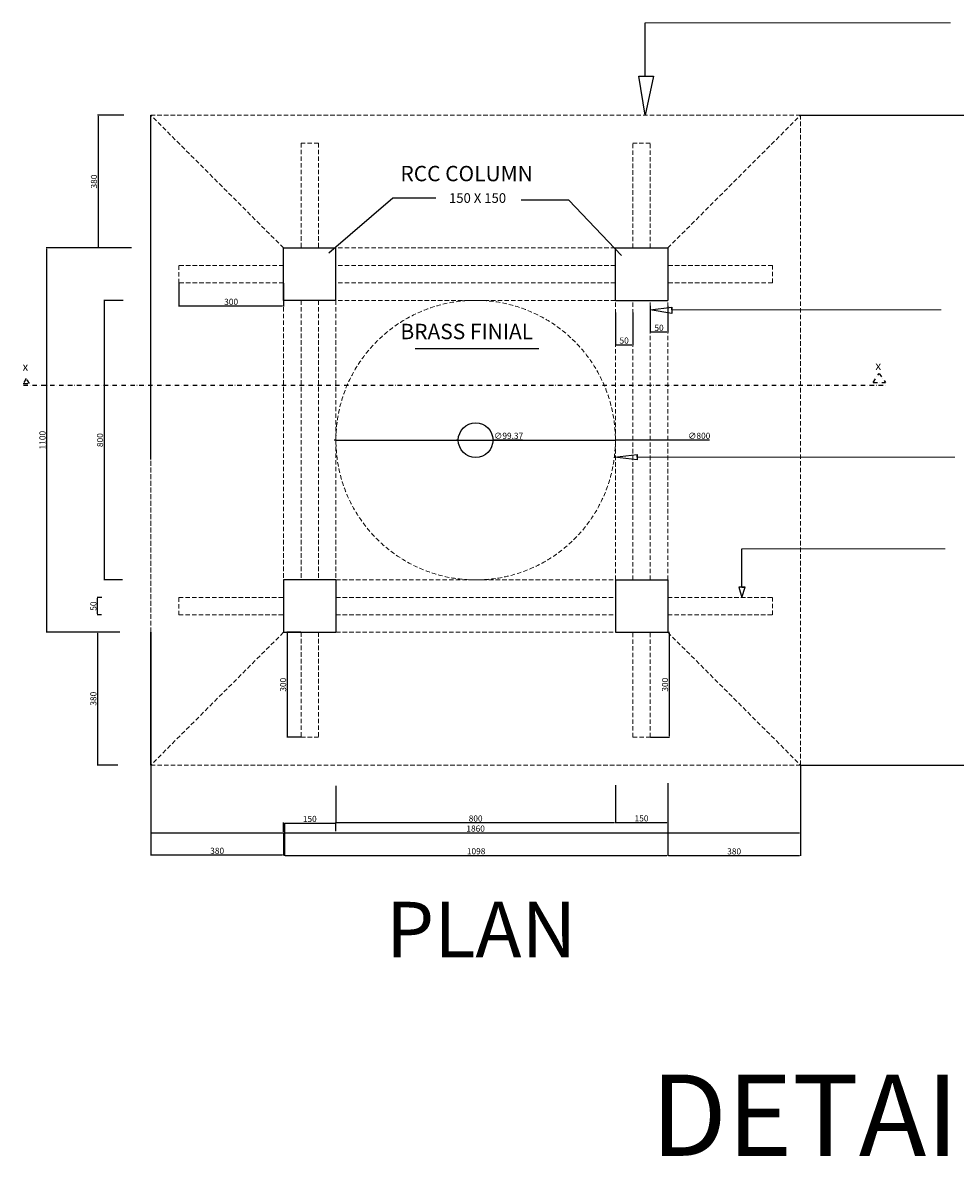
# Model space of a CAD drawing. Units: millimetres. Extents: x 498 to 8860, y -426 to 8717.
# Tile 1 of 9: x 498 to 3168, y -426 to 2821. Entities that reach past the tile are written whole.
import ezdxf

# ---------------------------------------------------------------- set-up
doc = ezdxf.new("R2010")
doc.units = ezdxf.units.MM
doc.linetypes.add('DASHDOT', pattern=[25.4, 12.7, -6.35, 0, -6.35])
doc.linetypes.add('DASHED', pattern=[19.05, 12.7, -6.35])
for name, color, linetype, lineweight in [('A-ANNO-DIMS', 2, 'Continuous', 18), ('A-ANNO-SYMB', 1, 'DASHDOT', 25), ('A-ANNO-TEXT', 3, 'Continuous', 18), ('A-DETL', 7, 'Continuous', 25), ('A-DETL-OVHD', 8, 'DASHED', 18)]:
    doc.layers.add(name, color=color, linetype=linetype, lineweight=lineweight)
doc.styles.get("Standard").update_dxf_attribs({"font": 'arial.ttf'})
doc.dimstyles.new('ISO-25', dxfattribs={"dimtxt": 17.5, "dimasz": 2.5, "dimexe": 1.25, "dimexo": 0.625, "dimtad": 1, "dimdec": 0, "dimtxsty": 'Standard', "dimcen": 2.5, "dimadec": 0, "dimazin": 0, "dimtfac": 1, "dimtdec": 0, "dimtmove": 0, "dimatfit": 3, "dimfxl": 1, "dimarcsym": 0})

# ---------------------------------------------------------------- blocks, each defined once
blk = doc.blocks.new('*D1')
at = {"layer": 'A-ANNO-DIMS', "color": 0, "lineweight": -2, "transparency": 16777216}
for p, q in [((944.7, 2075.6), (944.7, 2009.1)), ((1244.7, 2075.6), (1244.7, 2009.1)), ((947.2, 2010.4), (1242.2, 2010.4))]:
    blk.add_line(p, q, dxfattribs=at)
at = {"layer": 'A-ANNO-DIMS', "color": 0, "transparency": 16777216}
for points in [[(947.2, 2010.8), (947.2, 2009.9), (944.7, 2010.4)], [(1242.2, 2010.8), (1242.2, 2009.9), (1244.7, 2010.4)]]:
    blk.add_solid(points, dxfattribs=at)
at = {"layer": 'Defpoints', "color": 0, "transparency": 16777216}
for p in [(944.7, 2076.3), (1244.7, 2076.3), (1244.7, 2010.4)]:
    blk.add_point(p, dxfattribs=at)
at = {"layer": 'A-ANNO-DIMS', "color": 0, "transparency": 16777216, "insert": (1094.7, 2019.9), "char_height": 17.5, "attachment_point": 5}
blk.add_mtext('300', dxfattribs=at)
blk = doc.blocks.new('*D2')
at = {"layer": 'A-ANNO-DIMS', "color": 0, "lineweight": -2, "transparency": 16777216}
for p, q in [((724.4, 1176.3), (710.9, 1176.3)), ((712.2, 1128.8), (712.2, 1173.8)), ((723.9, 1126.3), (710.9, 1126.3))]:
    blk.add_line(p, q, dxfattribs=at)
at = {"layer": 'A-ANNO-DIMS', "color": 0, "transparency": 16777216}
for points in [[(711.8, 1173.8), (712.6, 1173.8), (712.2, 1176.3)], [(711.8, 1128.8), (712.6, 1128.8), (712.2, 1126.3)]]:
    blk.add_solid(points, dxfattribs=at)
at = {"layer": 'Defpoints', "color": 0, "transparency": 16777216}
for p in [(712.2, 1176.3), (725, 1176.3), (724.5, 1126.3)]:
    blk.add_point(p, dxfattribs=at)
at = {"layer": 'A-ANNO-DIMS', "color": 0, "transparency": 16777216, "insert": (702.6, 1151.3), "char_height": 17.5, "attachment_point": 5, "rotation": 90}
blk.add_mtext('50', dxfattribs=at)
blk = doc.blocks.new('*D3')
at = {"layer": 'A-ANNO-DIMS', "color": 0, "lineweight": -2, "transparency": 16777216}
for p, q in [((787.7, 2556.3), (712.6, 2556.3)), ((713.9, 2553.8), (713.9, 2178.8)), ((809.4, 2176.3), (712.6, 2176.3))]:
    blk.add_line(p, q, dxfattribs=at)
at = {"layer": 'A-ANNO-DIMS', "color": 0, "transparency": 16777216}
for points in [[(713.4, 2553.8), (714.3, 2553.8), (713.9, 2556.3)], [(713.4, 2178.8), (714.3, 2178.8), (713.9, 2176.3)]]:
    blk.add_solid(points, dxfattribs=at)
at = {"layer": 'Defpoints', "color": 0, "transparency": 16777216}
for p in [(788.4, 2556.3), (713.9, 2176.3), (810, 2176.3)]:
    blk.add_point(p, dxfattribs=at)
at = {"layer": 'A-ANNO-DIMS', "color": 0, "transparency": 16777216, "insert": (704.3, 2366.3), "char_height": 17.5, "attachment_point": 5, "rotation": 90}
blk.add_mtext('380', dxfattribs=at)
blk = doc.blocks.new('*D4')
at = {"layer": 'A-ANNO-DIMS', "color": 0, "lineweight": -2, "transparency": 16777216}
for p, q in [((775.7, 1076.3), (710.9, 1076.3)), ((712.2, 1073.8), (712.2, 698.8)), ((770.5, 696.3), (710.9, 696.3))]:
    blk.add_line(p, q, dxfattribs=at)
at = {"layer": 'A-ANNO-DIMS', "color": 0, "transparency": 16777216}
for points in [[(711.8, 1073.8), (712.6, 1073.8), (712.2, 1076.3)], [(711.8, 698.8), (712.6, 698.8), (712.2, 696.3)]]:
    blk.add_solid(points, dxfattribs=at)
at = {"layer": 'Defpoints', "color": 0, "transparency": 16777216}
for p in [(776.4, 1076.3), (712.2, 696.3), (771.2, 696.3)]:
    blk.add_point(p, dxfattribs=at)
at = {"layer": 'A-ANNO-DIMS', "color": 0, "transparency": 16777216, "insert": (702.6, 886.3), "char_height": 17.5, "attachment_point": 5, "rotation": 90}
blk.add_mtext('380', dxfattribs=at)
blk = doc.blocks.new('*D5')
at = {"layer": 'A-ANNO-DIMS', "color": 0, "lineweight": -2, "transparency": 16777216}
for p, q in [((739.8, 2176.3), (565.1, 2176.3)), ((566.3, 2173.8), (566.3, 1078.8)), ((775.7, 1076.3), (565.1, 1076.3))]:
    blk.add_line(p, q, dxfattribs=at)
at = {"layer": 'A-ANNO-DIMS', "color": 0, "transparency": 16777216}
for points in [[(565.9, 2173.8), (566.7, 2173.8), (566.3, 2176.3)], [(565.9, 1078.8), (566.7, 1078.8), (566.3, 1076.3)]]:
    blk.add_solid(points, dxfattribs=at)
at = {"layer": 'Defpoints', "color": 0, "transparency": 16777216}
for p in [(740.4, 2176.3), (566.3, 1076.3), (776.4, 1076.3)]:
    blk.add_point(p, dxfattribs=at)
at = {"layer": 'A-ANNO-DIMS', "color": 0, "transparency": 16777216, "insert": (556.8, 1626.3), "char_height": 17.5, "attachment_point": 5, "rotation": 90}
blk.add_mtext('1100', dxfattribs=at)
blk = doc.blocks.new('*D6')
at = {"layer": 'A-ANNO-DIMS', "color": 0, "lineweight": -2, "transparency": 16777216}
for p, q in [((1294.1, 1076.3), (1254, 1076.3)), ((1255.3, 1073.8), (1255.3, 778.8)), ((1294.1, 776.3), (1254, 776.3))]:
    blk.add_line(p, q, dxfattribs=at)
at = {"layer": 'A-ANNO-DIMS', "color": 0, "transparency": 16777216}
for points in [[(1254.9, 1073.8), (1255.7, 1073.8), (1255.3, 1076.3)], [(1254.9, 778.8), (1255.7, 778.8), (1255.3, 776.3)]]:
    blk.add_solid(points, dxfattribs=at)
at = {"layer": 'Defpoints', "color": 0, "transparency": 16777216}
for p in [(1294.7, 1076.3), (1255.3, 776.3), (1294.7, 776.3)]:
    blk.add_point(p, dxfattribs=at)
at = {"layer": 'A-ANNO-DIMS', "color": 0, "transparency": 16777216, "insert": (1245.7, 926.3), "char_height": 17.5, "attachment_point": 5, "rotation": 90}
blk.add_mtext('300', dxfattribs=at)
blk = doc.blocks.new('*D7')
at = {"layer": 'A-ANNO-DIMS', "color": 0, "lineweight": -2, "transparency": 16777216}
for p, q in [((2295.4, 1076.3), (2349.9, 1076.3)), ((2348.6, 1073.8), (2348.6, 778.8)), ((2295.4, 776.3), (2349.9, 776.3))]:
    blk.add_line(p, q, dxfattribs=at)
at = {"layer": 'A-ANNO-DIMS', "color": 0, "transparency": 16777216}
for points in [[(2348.2, 1073.8), (2349, 1073.8), (2348.6, 1076.3)], [(2348.2, 778.8), (2349, 778.8), (2348.6, 776.3)]]:
    blk.add_solid(points, dxfattribs=at)
at = {"layer": 'Defpoints', "color": 0, "transparency": 16777216}
for p in [(2294.7, 1076.3), (2294.7, 776.3), (2348.6, 776.3)]:
    blk.add_point(p, dxfattribs=at)
at = {"layer": 'A-ANNO-DIMS', "color": 0, "transparency": 16777216, "insert": (2339.1, 926.3), "char_height": 17.5, "attachment_point": 5, "rotation": 90}
blk.add_mtext('300', dxfattribs=at)
blk = doc.blocks.new('*D8')
at = {"layer": 'A-ANNO-DIMS', "color": 0, "lineweight": -2, "transparency": 16777216}
for p, q in [((2294.7, 2010.9), (2294.7, 1934.6)), ((2344.7, 2010.9), (2344.7, 1934.6)), ((2297.2, 1935.9), (2342.2, 1935.9))]:
    blk.add_line(p, q, dxfattribs=at)
at = {"layer": 'A-ANNO-DIMS', "color": 0, "transparency": 16777216}
for points in [[(2297.2, 1936.3), (2297.2, 1935.4), (2294.7, 1935.9)], [(2342.2, 1936.3), (2342.2, 1935.4), (2344.7, 1935.9)]]:
    blk.add_solid(points, dxfattribs=at)
at = {"layer": 'Defpoints', "color": 0, "transparency": 16777216}
for p in [(2294.7, 2011.5), (2344.7, 2011.5), (2344.7, 1935.9)]:
    blk.add_point(p, dxfattribs=at)
at = {"layer": 'A-ANNO-DIMS', "color": 0, "transparency": 16777216, "insert": (2319.7, 1945.4), "char_height": 17.5, "attachment_point": 5}
blk.add_mtext('50', dxfattribs=at)
blk = doc.blocks.new('*D9')
at = {"layer": 'A-ANNO-DIMS', "color": 0, "lineweight": -2, "transparency": 16777216}
for p, q in [((2194.7, 1991.4), (2194.7, 1898.2)), ((2244.7, 1991.4), (2244.7, 1898.2)), ((2197.2, 1899.5), (2242.2, 1899.5))]:
    blk.add_line(p, q, dxfattribs=at)
at = {"layer": 'A-ANNO-DIMS', "color": 0, "transparency": 16777216}
for points in [[(2197.2, 1899.9), (2197.2, 1899.1), (2194.7, 1899.5)], [(2242.2, 1899.9), (2242.2, 1899.1), (2244.7, 1899.5)]]:
    blk.add_solid(points, dxfattribs=at)
at = {"layer": 'Defpoints', "color": 0, "transparency": 16777216}
for p in [(2194.7, 1992.1), (2244.7, 1992.1), (2244.7, 1899.5)]:
    blk.add_point(p, dxfattribs=at)
at = {"layer": 'A-ANNO-DIMS', "color": 0, "transparency": 16777216, "insert": (2219.7, 1909), "char_height": 17.5, "attachment_point": 5}
blk.add_mtext('50', dxfattribs=at)
blk = doc.blocks.new('*D10')
at = {"layer": 'A-ANNO-DIMS', "color": 0, "lineweight": -2, "transparency": 16777216}
for p, q in [((785.3, 2026.3), (730, 2026.3)), ((731.3, 2023.8), (731.3, 1228.8)), ((783.7, 1226.3), (730, 1226.3))]:
    blk.add_line(p, q, dxfattribs=at)
at = {"layer": 'A-ANNO-DIMS', "color": 0, "transparency": 16777216}
for points in [[(730.8, 2023.8), (731.7, 2023.8), (731.3, 2026.3)], [(730.8, 1228.8), (731.7, 1228.8), (731.3, 1226.3)]]:
    blk.add_solid(points, dxfattribs=at)
at = {"layer": 'Defpoints', "color": 0, "transparency": 16777216}
for p in [(785.9, 2026.3), (731.3, 1226.3), (784.3, 1226.3)]:
    blk.add_point(p, dxfattribs=at)
at = {"layer": 'A-ANNO-DIMS', "color": 0, "transparency": 16777216, "insert": (721.7, 1626.3), "char_height": 17.5, "attachment_point": 5, "rotation": 90}
blk.add_mtext('800', dxfattribs=at)
blk = doc.blocks.new('*D11')
at = {"layer": 'A-ANNO-DIMS', "color": 0, "lineweight": -2, "transparency": 16777216}
for p, q in [((864.7, 502.8), (864.7, 437.9)), ((1244.7, 503.5), (1244.7, 437.9)), ((867.2, 439.1), (1242.2, 439.1))]:
    blk.add_line(p, q, dxfattribs=at)
at = {"layer": 'A-ANNO-DIMS', "color": 0, "transparency": 16777216}
for points in [[(867.2, 439.5), (867.2, 438.7), (864.7, 439.1)], [(1242.2, 439.5), (1242.2, 438.7), (1244.7, 439.1)]]:
    blk.add_solid(points, dxfattribs=at)
at = {"layer": 'Defpoints', "color": 0, "transparency": 16777216}
for p in [(864.7, 503.4), (1244.7, 504.2), (1244.7, 439.1)]:
    blk.add_point(p, dxfattribs=at)
at = {"layer": 'A-ANNO-DIMS', "color": 0, "transparency": 16777216, "insert": (1054.7, 448.7), "char_height": 17.5, "attachment_point": 5}
blk.add_mtext('380', dxfattribs=at)
blk = doc.blocks.new('*D12')
at = {"layer": 'A-ANNO-DIMS', "color": 0, "lineweight": -2, "transparency": 16777216}
for p, q in [((1244.7, 504.8), (1244.7, 531.6)), ((1247.2, 530.3), (1392.2, 530.3)), ((1394.7, 506.7), (1394.7, 531.6))]:
    blk.add_line(p, q, dxfattribs=at)
at = {"layer": 'A-ANNO-DIMS', "color": 0, "transparency": 16777216}
for points in [[(1247.2, 530.7), (1247.2, 529.9), (1244.7, 530.3)], [(1392.2, 530.7), (1392.2, 529.9), (1394.7, 530.3)]]:
    blk.add_solid(points, dxfattribs=at)
at = {"layer": 'Defpoints', "color": 0, "transparency": 16777216}
for p in [(1394.7, 530.3), (1244.7, 504.2), (1394.7, 506)]:
    blk.add_point(p, dxfattribs=at)
at = {"layer": 'A-ANNO-DIMS', "color": 0, "transparency": 16777216, "insert": (1319.7, 539.9), "char_height": 17.5, "attachment_point": 5}
blk.add_mtext('150', dxfattribs=at)
blk = doc.blocks.new('*D13')
at = {"layer": 'A-ANNO-DIMS', "color": 0, "lineweight": -2, "transparency": 16777216}
for p, q in [((1394.7, 636.9), (1394.7, 530.3)), ((2194.7, 639.2), (2194.7, 530.3)), ((1397.2, 531.6), (2192.2, 531.6))]:
    blk.add_line(p, q, dxfattribs=at)
at = {"layer": 'A-ANNO-DIMS', "color": 0, "transparency": 16777216}
for points in [[(1397.2, 532), (1397.2, 531.1), (1394.7, 531.6)], [(2192.2, 532), (2192.2, 531.1), (2194.7, 531.6)]]:
    blk.add_solid(points, dxfattribs=at)
at = {"layer": 'Defpoints', "color": 0, "transparency": 16777216}
for p in [(1394.7, 637.5), (2194.7, 639.9), (2194.7, 531.6)]:
    blk.add_point(p, dxfattribs=at)
at = {"layer": 'A-ANNO-DIMS', "color": 0, "transparency": 16777216, "insert": (1794.7, 541.1), "char_height": 17.5, "attachment_point": 5}
blk.add_mtext('800', dxfattribs=at)
blk = doc.blocks.new('*D14')
at = {"layer": 'A-ANNO-DIMS', "color": 0, "lineweight": -2, "transparency": 16777216}
for p, q in [((2194.7, 614.7), (2194.7, 530.7)), ((2344.7, 605.3), (2344.7, 530.7)), ((2197.2, 532), (2342.2, 532))]:
    blk.add_line(p, q, dxfattribs=at)
at = {"layer": 'A-ANNO-DIMS', "color": 0, "transparency": 16777216}
for points in [[(2197.2, 532.4), (2197.2, 531.6), (2194.7, 532)], [(2342.2, 532.4), (2342.2, 531.6), (2344.7, 532)]]:
    blk.add_solid(points, dxfattribs=at)
at = {"layer": 'Defpoints', "color": 0, "transparency": 16777216}
for p in [(2194.7, 615.3), (2344.7, 605.9), (2344.7, 532)]:
    blk.add_point(p, dxfattribs=at)
at = {"layer": 'A-ANNO-DIMS', "color": 0, "transparency": 16777216, "insert": (2269.7, 541.5), "char_height": 17.5, "attachment_point": 5}
blk.add_mtext('150', dxfattribs=at)
blk = doc.blocks.new('*D15')
at = {"layer": 'A-ANNO-DIMS', "color": 0, "lineweight": -2, "transparency": 16777216}
for p, q in [((2344.7, 592.2), (2344.7, 436.6)), ((1247.2, 529.3), (1247.2, 436.6)), ((1249.7, 437.9), (2342.2, 437.9))]:
    blk.add_line(p, q, dxfattribs=at)
at = {"layer": 'A-ANNO-DIMS', "color": 0, "transparency": 16777216}
for points in [[(1249.7, 438.3), (1249.7, 437.5), (1247.2, 437.9)], [(2342.2, 438.3), (2342.2, 437.5), (2344.7, 437.9)]]:
    blk.add_solid(points, dxfattribs=at)
at = {"layer": 'Defpoints', "color": 0, "transparency": 16777216}
for p in [(2344.7, 592.9), (1247.2, 529.9), (2344.7, 437.9)]:
    blk.add_point(p, dxfattribs=at)
at = {"layer": 'A-ANNO-DIMS', "color": 0, "transparency": 16777216, "insert": (1796, 447.4), "char_height": 17.5, "attachment_point": 5}
blk.add_mtext('1098', dxfattribs=at)
blk = doc.blocks.new('*D16')
at = {"layer": 'A-ANNO-DIMS', "color": 0, "lineweight": -2, "transparency": 16777216}
for p, q in [((2344.7, 644.1), (2344.7, 436.2)), ((2724.7, 520.1), (2724.7, 436.2)), ((2347.2, 437.5), (2722.2, 437.5))]:
    blk.add_line(p, q, dxfattribs=at)
at = {"layer": 'A-ANNO-DIMS', "color": 0, "transparency": 16777216}
for points in [[(2347.2, 437.9), (2347.2, 437), (2344.7, 437.5)], [(2722.2, 437.9), (2722.2, 437), (2724.7, 437.5)]]:
    blk.add_solid(points, dxfattribs=at)
at = {"layer": 'Defpoints', "color": 0, "transparency": 16777216}
for p in [(2344.7, 644.7), (2724.7, 520.8), (2724.7, 437.5)]:
    blk.add_point(p, dxfattribs=at)
at = {"layer": 'A-ANNO-DIMS', "color": 0, "transparency": 16777216, "insert": (2534.7, 447), "char_height": 17.5, "attachment_point": 5}
blk.add_mtext('380', dxfattribs=at)
blk = doc.blocks.new('*D64')
at = {"layer": 'A-ANNO-DIMS', "color": 0, "lineweight": -2, "transparency": 16777216}
for p, q in [((864.7, 695.6), (864.7, 501.5)), ((2724.7, 695.6), (2724.7, 501.5)), ((867.2, 502.8), (2722.2, 502.8))]:
    blk.add_line(p, q, dxfattribs=at)
at = {"layer": 'A-ANNO-DIMS', "color": 0, "transparency": 16777216}
for points in [[(867.2, 503.2), (867.2, 502.4), (864.7, 502.8)], [(2722.2, 503.2), (2722.2, 502.4), (2724.7, 502.8)]]:
    blk.add_solid(points, dxfattribs=at)
at = {"layer": 'Defpoints', "color": 0, "transparency": 16777216}
for p in [(864.7, 696.3), (2724.7, 696.3), (2724.7, 502.8)]:
    blk.add_point(p, dxfattribs=at)
at = {"layer": 'A-ANNO-DIMS', "color": 0, "transparency": 16777216, "insert": (1794.7, 512.3), "char_height": 17.5, "attachment_point": 5}
blk.add_mtext('1860', dxfattribs=at)
blk = doc.blocks.new('*D65')
at = {"layer": 'A-ANNO-DIMS', "color": 0, "lineweight": -2, "transparency": 16777216}
for p, q in [((2725.4, 2556.3), (3361, 2556.3)), ((3359.7, 698.8), (3359.7, 2553.8)), ((2725.4, 696.3), (3361, 696.3))]:
    blk.add_line(p, q, dxfattribs=at)
at = {"layer": 'A-ANNO-DIMS', "color": 0, "transparency": 16777216}
for points in [[(3359.3, 2553.8), (3360.1, 2553.8), (3359.7, 2556.3)], [(3359.3, 698.8), (3360.1, 698.8), (3359.7, 696.3)]]:
    blk.add_solid(points, dxfattribs=at)
at = {"layer": 'Defpoints', "color": 0, "transparency": 16777216}
for p in [(2724.7, 2556.3), (3359.7, 2556.3), (2724.7, 696.3)]:
    blk.add_point(p, dxfattribs=at)
at = {"layer": 'A-ANNO-DIMS', "color": 0, "transparency": 16777216, "insert": (3350.2, 1626.3), "char_height": 17.5, "attachment_point": 5, "rotation": 90}
blk.add_mtext('1860', dxfattribs=at)
blk = doc.blocks.new('*D84')
at = {"layer": 'A-ANNO-DIMS', "color": 0, "lineweight": -2, "transparency": 16777216}
for p, q in [((1392.2, 1626.2), (1389.7, 1626.2)), ((1394.7, 1626.2), (2194.7, 1626.3)), ((2464.2, 1626.3), (2197.2, 1626.3))]:
    blk.add_line(p, q, dxfattribs=at)
at = {"layer": 'A-ANNO-DIMS', "color": 0, "transparency": 16777216}
for points in [[(1392.2, 1626.7), (1392.2, 1625.8), (1394.7, 1626.2)], [(2197.2, 1626.7), (2197.2, 1625.9), (2194.7, 1626.3)]]:
    blk.add_solid(points, dxfattribs=at)
at = {"layer": 'Defpoints', "color": 0, "transparency": 16777216}
for p in [(1394.7, 1626.2), (2194.7, 1626.3)]:
    blk.add_point(p, dxfattribs=at)
at = {"layer": 'A-ANNO-DIMS', "color": 0, "transparency": 16777216, "insert": (2434.7, 1636.4), "char_height": 17.5, "attachment_point": 5, "rotation": 0.0041}
blk.add_mtext('∅800', dxfattribs=at)
blk = doc.blocks.new('*D85')
at = {"layer": 'A-ANNO-DIMS', "color": 0, "lineweight": -2, "transparency": 16777216}
for p, q in [((1742.5, 1626.2), (1740, 1626.2)), ((1745, 1626.2), (1844.4, 1626.3)), ((1928.8, 1626.3), (1846.9, 1626.3))]:
    blk.add_line(p, q, dxfattribs=at)
at = {"layer": 'A-ANNO-DIMS', "color": 0, "transparency": 16777216}
for points in [[(1742.5, 1626.7), (1742.5, 1625.8), (1745, 1626.2)], [(1846.9, 1626.7), (1846.9, 1625.9), (1844.4, 1626.3)]]:
    blk.add_solid(points, dxfattribs=at)
at = {"layer": 'Defpoints', "color": 0, "transparency": 16777216}
for p in [(1745, 1626.2), (1844.4, 1626.3)]:
    blk.add_point(p, dxfattribs=at)
at = {"layer": 'A-ANNO-DIMS', "color": 0, "transparency": 16777216, "insert": (1889.1, 1636.4), "char_height": 17.5, "attachment_point": 5, "rotation": 0.0327}
blk.add_mtext('∅99.37', dxfattribs=at)

msp = doc.modelspace()

# ---------------------------------------------------------------- linework, layer by layer
at = {"layer": 'A-ANNO-SYMB'}
for p, q in [((508.28, 1802.5), (499.782, 1788.76)), ((499.782, 1788.76), (517.675, 1788.76)), ((517.675, 1788.76), (508.28, 1802.5)), ((2932.339, 1791.292), (2949.582, 1817.301)), ((2932.339, 1791.292), (2968.288, 1791.292)), ((2949.582, 1817.301), (2968.288, 1791.292)), ((500.172, 1783.423), (2969.012, 1783.423))]:
    msp.add_line(p, q, dxfattribs=at)
at = {"layer": 'A-ANNO-TEXT'}
for p, q in [((2280.163, 2821.025), (3153.633, 2821.025)), ((2356.431, 1999.238), (3127.588, 1999.238)), ((2256.646, 1577.354), (3166.223, 1577.354)), ((2556.864, 1315.589), (3139.06, 1315.589))]:
    msp.add_line(p, q, dxfattribs=at)
at = {"layer": 'A-DETL'}
for p, q in [((2280.163, 2667.519), (2280.163, 2821.025)), ((2262.191, 2667.519), (2304.021, 2667.519)), ((2280.163, 2556.272), (2262.191, 2667.519)), ((2304.021, 2667.519), (2280.163, 2556.272)), ((1374.825, 2162.624), (1557.809, 2320.001)), ((1557.809, 2320.001), (1680.71, 2320.001)), ((2061.272, 2312.744), (1924.795, 2312.744)), ((2212.243, 2154.722), (2061.272, 2312.744)), ((1244.726, 2026.272), (1244.726, 2176.272)), ((1244.726, 2176.272), (1394.726, 2176.272)), ((1394.726, 2026.272), (1394.726, 2176.272)), ((2194.726, 2176.272), (2344.726, 2176.272)), ((2194.726, 2026.272), (2194.726, 2176.272)), ((2344.726, 2176.272), (2344.726, 2026.272)), ((1394.726, 2026.272), (1244.726, 2026.272)), ((2194.726, 2026.272), (2344.726, 2026.272)), ((2294.726, 1999.238), (2356.431, 2007.236)), ((2356.431, 1988.834), (2294.726, 1999.238)), ((2356.431, 1999.238), (2356.431, 2007.236)), ((2356.431, 2007.236), (2356.431, 1988.834)), ((1621.385, 1888.913), (1975.941, 1888.913)), ((2191.723, 1577.354), (2194.726, 1577.354)), ((2191.749, 1577.565), (2256.646, 1585.279)), ((2256.646, 1569.604), (2191.749, 1577.565)), ((2256.646, 1577.354), (2256.646, 1585.279)), ((2256.646, 1585.279), (2256.646, 1569.604)), ((2556.864, 1205.48), (2556.864, 1315.589)), ((1244.726, 1226.272), (1244.726, 1076.272)), ((1394.726, 1226.272), (1244.726, 1226.272)), ((1394.726, 1226.272), (1394.726, 1076.272)), ((2194.726, 1226.272), (2194.726, 1076.272)), ((2194.726, 1226.272), (2344.726, 1226.272)), ((2344.726, 1226.272), (2344.726, 1076.272)), ((2566.126, 1205.48), (2547.874, 1205.48)), ((2547.874, 1205.48), (2556.864, 1176.272)), ((2556.864, 1205.48), (2566.126, 1205.48)), ((2556.864, 1176.272), (2566.126, 1205.48)), ((864.726, 1076.272), (864.726, 696.272)), ((864.726, 1076.272), (864.726, 696.272)), ((864.726, 696.272), (864.726, 1076.272)), ((1244.726, 1076.272), (1394.726, 1076.272)), ((2194.726, 1076.272), (2344.726, 1076.272))]:
    msp.add_line(p, q, dxfattribs=at)
msp.add_lwpolyline([(864.726, 1570.972), (864.726, 2556.272)], dxfattribs=at)
msp.add_circle((1794.726, 1626.272), 49.685, dxfattribs=at)
at = {"layer": 'A-DETL-OVHD'}
for p, q in [((2724.726, 2556.272), (864.726, 2556.272)), ((864.726, 2556.272), (864.726, 696.272)), ((1244.726, 2176.272), (864.726, 2556.272)), ((2344.726, 2176.272), (2724.726, 2556.272)), ((2724.726, 696.272), (2724.726, 2556.272)), ((1294.726, 2476.272), (1294.726, 2176.272)), ((1344.726, 2476.272), (1294.726, 2476.272)), ((1344.726, 2476.272), (1344.726, 2176.272)), ((2244.726, 2176.272), (2244.726, 2476.272)), ((2294.726, 2476.272), (2244.726, 2476.272)), ((2294.726, 2176.272), (2294.726, 2476.272)), ((864.726, 2176.272), (864.726, 1076.272)), ((864.726, 1076.272), (864.726, 2176.272)), ((864.726, 1076.272), (864.726, 2176.272)), ((2194.726, 2176.272), (1394.726, 2176.272)), ((1244.726, 2126.272), (944.726, 2126.272)), ((944.726, 2126.272), (944.726, 2076.272)), ((2194.726, 2126.272), (1394.726, 2126.272)), ((2644.726, 2126.272), (2344.726, 2126.272)), ((2644.726, 2076.272), (2644.726, 2126.272)), ((1244.726, 2076.272), (944.726, 2076.272)), ((2194.726, 2076.272), (1394.726, 2076.272)), ((2644.726, 2076.272), (2344.726, 2076.272)), ((1244.726, 2026.272), (1244.726, 1226.272)), ((1294.726, 2026.272), (1294.726, 1226.272)), ((1344.726, 2026.272), (1344.726, 1226.272)), ((1394.726, 2026.272), (1394.726, 1226.272)), ((2194.726, 2026.272), (1394.726, 2026.272)), ((2194.726, 1226.272), (2194.726, 2026.272)), ((2244.726, 1226.272), (2244.726, 2026.272)), ((2294.726, 1226.272), (2294.726, 2026.272)), ((2344.726, 1226.272), (2344.726, 2026.272)), ((1394.726, 1226.272), (2194.726, 1226.272)), ((944.726, 1176.272), (1244.726, 1176.272)), ((944.726, 1176.272), (944.726, 1126.272)), ((1394.726, 1176.272), (2194.726, 1176.272)), ((2344.726, 1176.272), (2644.726, 1176.272)), ((2644.726, 1126.272), (2644.726, 1176.272)), ((944.726, 1126.272), (1244.726, 1126.272)), ((1394.726, 1126.272), (2194.726, 1126.272)), ((2344.726, 1126.272), (2644.726, 1126.272)), ((1244.726, 1076.272), (864.726, 696.272)), ((1294.726, 1076.272), (1294.726, 776.272)), ((1344.726, 1076.272), (1344.726, 776.272)), ((1394.726, 1076.272), (2344.726, 1076.272)), ((2244.726, 776.272), (2244.726, 1076.272)), ((2294.726, 776.272), (2294.726, 1076.272)), ((2344.726, 1076.272), (2724.726, 696.272)), ((1294.726, 776.272), (1344.726, 776.272)), ((2244.726, 776.272), (2294.726, 776.272)), ((864.726, 696.272), (2724.726, 696.272))]:
    msp.add_line(p, q, dxfattribs=at)
msp.add_circle((1794.726, 1626.272), 400, dxfattribs=at)

# ---------------------------------------------------------------- texts
at = {"layer": 'A-ANNO-TEXT'}
for s, height, p in [('RCC COLUMN', 43.9996, (1579.332, 2367.205)), ('150 X 150', 27.5323, (1718.418, 2305.409)), ('BRASS FINIAL', 43.99963, (1579.332, 1915.179)), ('x', 24.132, (497.481, 1824.626)), ('x', 24.132, (2939.066, 1827.157)), ('PLAN', 159.2, (1538.504, 145.767)), ('DETAIL OF CHATTRI', 232.82067, (2295.778, -422.188))]:
    msp.add_text(s, height=height, dxfattribs=at).set_placement(p)

# ---------------------------------------------------------------- dimensions: what is measured, and where the dimension line sits
at = {"layer": 'A-ANNO-DIMS'}
for base, p1, p2, override, picture, middle in [((713.859, 2176.272), (788.355, 2556.272), (810.028, 2176.272), {"dimclrd": 0, "dimclre": 0, "dimclrt": 0}, '*D3', (704.293, 2366.272)), ((3359.723, 2556.272), (2724.726, 696.272), (2724.726, 2556.272), {"dimdec": 0, "dimlfac": 1, "dimrnd": 0, "dimzin": 0, "dimdsep": 46, "dimlunit": 2}, '*D65', (3350.163, 1626.272)), ((566.318, 1076.272), (740.438, 2176.272), (776.358, 1076.272), {"dimclrd": 0, "dimclre": 0, "dimclrt": 0}, '*D5', (556.758, 1626.272)), ((731.252, 1226.272), (785.875, 2026.272), (784.318, 1226.272), {"dimclrd": 0, "dimclre": 0, "dimclrt": 0}, '*D10', (721.692, 1626.272)), ((712.193, 1176.272), (724.515, 1126.272), (725, 1176.272), {"dimclrd": 0, "dimclre": 0, "dimclrt": 0}, '*D2', (702.633, 1151.272)), ((712.193, 696.272), (776.358, 1076.272), (771.173, 696.272), {"dimclrd": 0, "dimclre": 0, "dimclrt": 0}, '*D4', (702.627, 886.272)), ((1255.292, 776.272), (1294.726, 1076.272), (1294.726, 776.272), {"dimclrd": 0, "dimclre": 0, "dimclrt": 0}, '*D6', (1245.726, 926.272)), ((2348.619, 776.272), (2294.726, 1076.272), (2294.726, 776.272), {"dimclrd": 0, "dimclre": 0, "dimclrt": 0}, '*D7', (2339.053, 926.272))]:
    dim = msp.add_linear_dim(base=base, p1=p1, p2=p2, angle=90, dimstyle='ISO-25', override=override, dxfattribs=at)
    dim.commit()
    dim.dimension.update_dxf_attribs({"geometry": picture, "text_midpoint": middle})
for base, p1, p2, override, picture, middle in [((1244.726, 2010.363), (944.726, 2076.272), (1244.726, 2076.272), {"dimclrd": 0, "dimclre": 0, "dimclrt": 0}, '*D1', (1094.726, 2019.929)), ((2244.726, 1899.48), (2194.726, 1992.073), (2244.726, 1992.073), {"dimclrd": 0, "dimclre": 0, "dimclrt": 0}, '*D9', (2219.726, 1909.04)), ((2344.726, 1935.864), (2294.726, 2011.524), (2344.726, 2011.524), {"dimclrd": 0, "dimclre": 0, "dimclrt": 0}, '*D8', (2319.726, 1945.424)), ((2724.726, 502.772), (864.726, 696.272), (2724.726, 696.272), {"dimdec": 0, "dimlfac": 1, "dimrnd": 0, "dimzin": 0, "dimdsep": 46, "dimlunit": 2}, '*D64', (1794.726, 512.332)), ((2194.726, 531.552), (1394.726, 637.483), (2194.726, 639.862), {"dimclrd": 0, "dimclre": 0, "dimclrt": 0}, '*D13', (1794.726, 541.112)), ((2724.726, 437.453), (2344.726, 644.702), (2724.726, 520.751), {"dimclrd": 0, "dimclre": 0, "dimclrt": 0}, '*D16', (2534.726, 447.019)), ((2344.725950073, 437.869376506), (1247.225950073, 529.88568661), (2344.725950073, 592.870168718), {"dimclrd": 0, "dimclre": 0, "dimclrt": 0}, '*D15', (1795.975950073, 447.429403791)), ((2344.726, 531.969), (2194.726, 615.279), (2344.726, 605.925), {"dimclrd": 0, "dimclre": 0, "dimclrt": 0}, '*D14', (2269.726, 541.529)), ((1394.726, 530.302), (1244.726, 504.158), (1394.726, 506.049), {"dimclrd": 0, "dimclre": 0, "dimclrt": 0}, '*D12', (1319.726, 539.862)), ((1244.726, 439.119), (864.726, 503.435), (1244.726, 504.158), {"dimclrd": 0, "dimclre": 0, "dimclrt": 0}, '*D11', (1054.726, 448.685))]:
    dim = msp.add_linear_dim(base=base, p1=p1, p2=p2, dimstyle='ISO-25', override=override, dxfattribs=at)
    dim.commit()
    dim.dimension.update_dxf_attribs({"geometry": picture, "text_midpoint": middle})
for p1, p2, override, picture, middle in [((1394.726, 1626.243), (2194.726, 1626.3), {"dimdec": 0, "dimlfac": 1, "dimrnd": 0, "dimzin": 0, "dimdsep": 46, "dimlunit": 2}, '*D84', (2434.726, 1626.317)), ((1745.041, 1626.243), (1844.411, 1626.3), {"dimdec": 2, "dimlfac": 1, "dimrnd": 0, "dimzin": 0, "dimdsep": 46, "dimlunit": 2}, '*D85', (1889.083, 1626.326))]:
    dim = msp.add_diameter_dim_2p(p1=p1, p2=p2, dimstyle='ISO-25', override=override, dxfattribs=at)
    dim.commit()
    dim.dimension.update_dxf_attribs({"geometry": picture, "text_midpoint": middle, "dimtype": 163})

doc.saveas('drawing.dxf')
